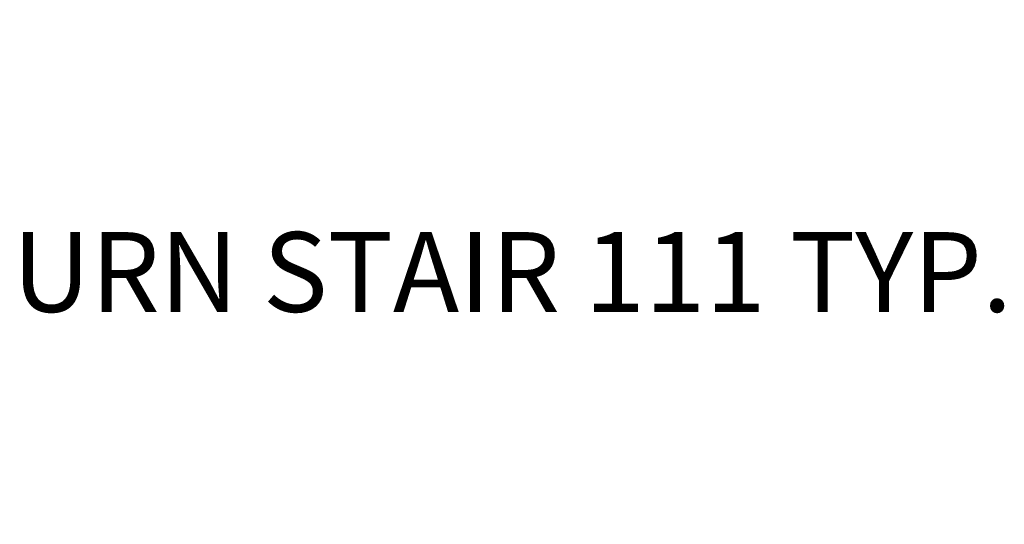
# Model space of a CAD drawing. Units: inches. Extents: x 73 to 1216, y -495 to 328.
# Tile 7 of 9: x 994 to 1216, y -495 to -382. Entities that reach past the tile are written whole.
import ezdxf

# ---------------------------------------------------------------- set-up
doc = ezdxf.new("R2010")
doc.units = ezdxf.units.IN
doc.layers.add('A-ANNO-DIMS', color=2, linetype='Continuous', lineweight=18)
doc.styles.get("Standard").update_dxf_attribs({"font": 'arial.ttf'})
doc.dimstyles.get("Standard").update_dxf_attribs({"dimtxt": 18, "dimasz": 12, "dimexe": 0.18, "dimexo": 0.0625, "dimgap": 0.09, "dimtad": 0, "dimtih": 1, "dimtoh": 1, "dimdec": 0, "dimzin": 0, "dimdsep": 46, "dimlunit": 3, "dimtxsty": 'Standard', "dimcen": 0.09, "dimadec": 0, "dimazin": 0, "dimtfac": 1, "dimtdec": 0, "dimtofl": 0, "dimtmove": 0, "dimatfit": 3, "dimfxl": 1, "dimtolj": 1, "dimtzin": 0, "dimarcsym": 0})

# ---------------------------------------------------------------- blocks, each defined once
blk = doc.blocks.new('*D46')
at = {"layer": 'A-ANNO-DIMS', "color": 0, "lineweight": -2, "transparency": 16777216}
for p, q in [((813.16, -421.89), (813.16, -438.65)), ((924.16, -421.89), (924.16, -438.65)), ((825.16, -438.47), (912.16, -438.47)), ((924.16, -438.47), (936.16, -438.47))]:
    blk.add_line(p, q, dxfattribs=at)
at = {"layer": 'A-ANNO-DIMS', "color": 0, "transparency": 16777216}
for points in [[(825.16, -436.47), (825.16, -440.47), (813.16, -438.47)], [(912.16, -436.47), (912.16, -440.47), (924.16, -438.47)]]:
    blk.add_solid(points, dxfattribs=at)
at = {"layer": 'Defpoints', "color": 0, "transparency": 16777216}
for p in [(813.16, -421.82), (924.16, -421.82), (924.16, -438.47)]:
    blk.add_point(p, dxfattribs=at)
at = {"layer": 'A-ANNO-DIMS', "color": 0, "transparency": 16777216, "insert": (1082.99, -438.47), "char_height": 18, "attachment_point": 5}
blk.add_mtext('\\A1;RETURN STAIR 111 TYP.', dxfattribs=at)

msp = doc.modelspace()

# ---------------------------------------------------------------- dimensions: what is measured, and where the dimension line sits
at = {"layer": 'A-ANNO-DIMS'}
dim = msp.add_linear_dim(base=(924.1647, -438.4737), p1=(813.1647, -421.8237), p2=(924.1647, -421.8237), text='RETURN STAIR <> TYP.', dimstyle='Standard', override={"dimdec": 0, "dimlfac": 1, "dimrnd": 0, "dimzin": 0, "dimdsep": 46, "dimlunit": 2}, dxfattribs=at)
dim.commit()
dim.dimension.update_dxf_attribs({"geometry": '*D46', "text_midpoint": (1082.9866, -438.4737)})

doc.saveas('drawing.dxf')
